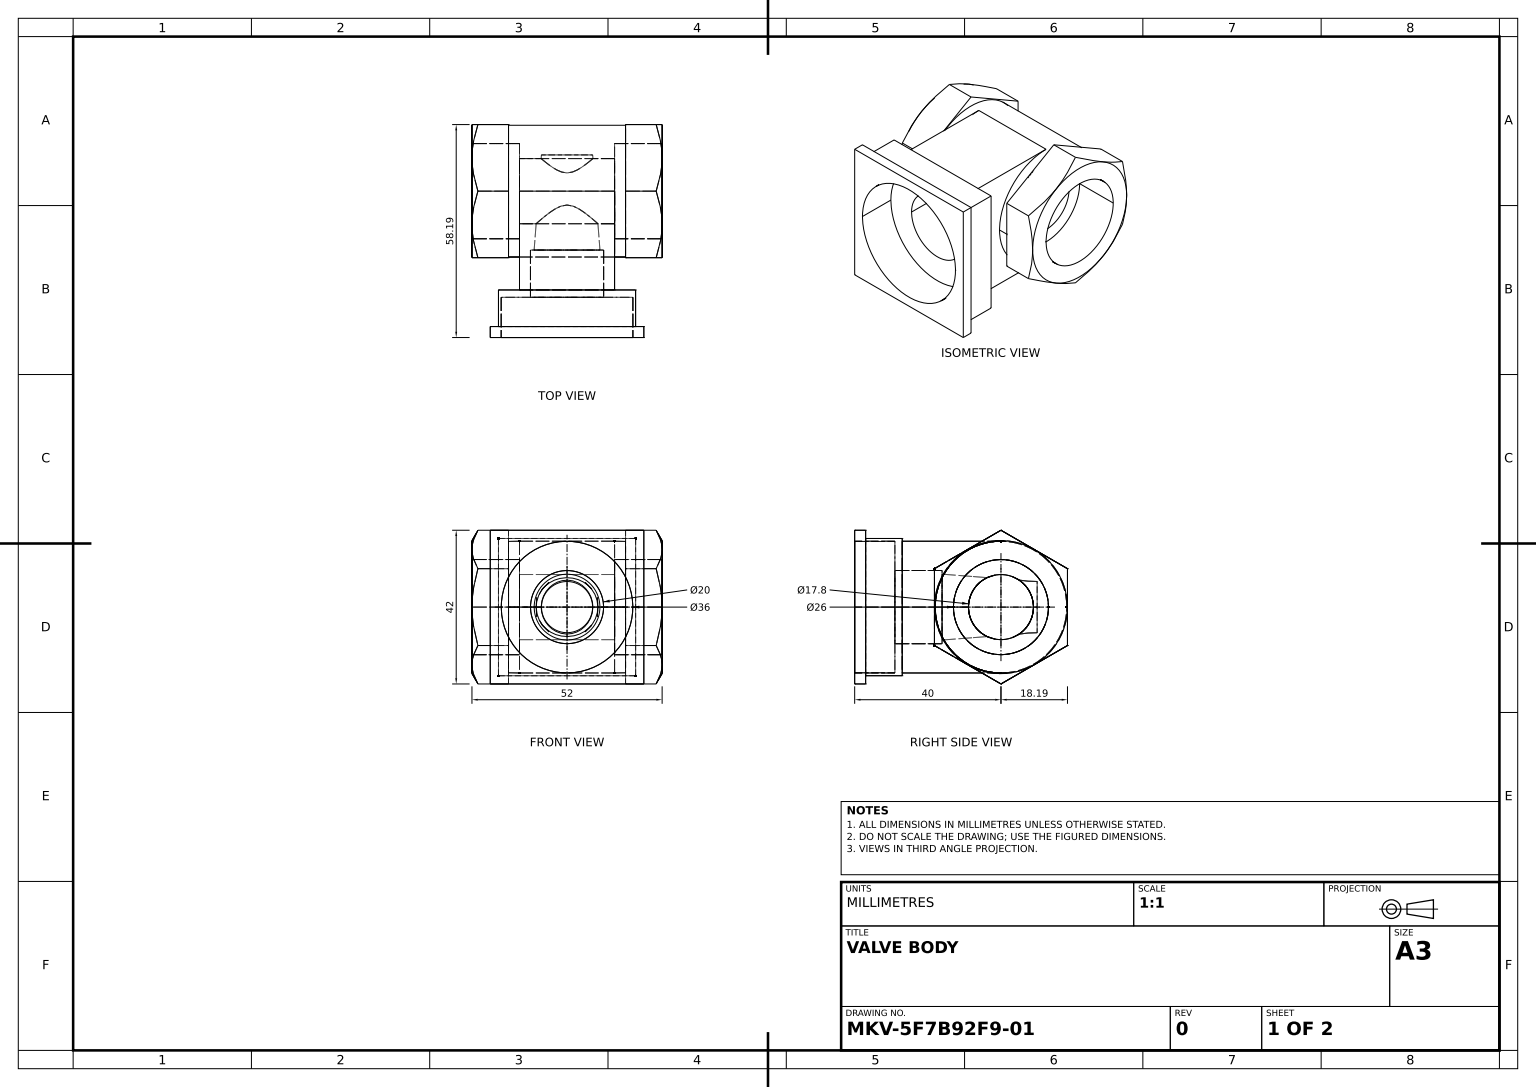
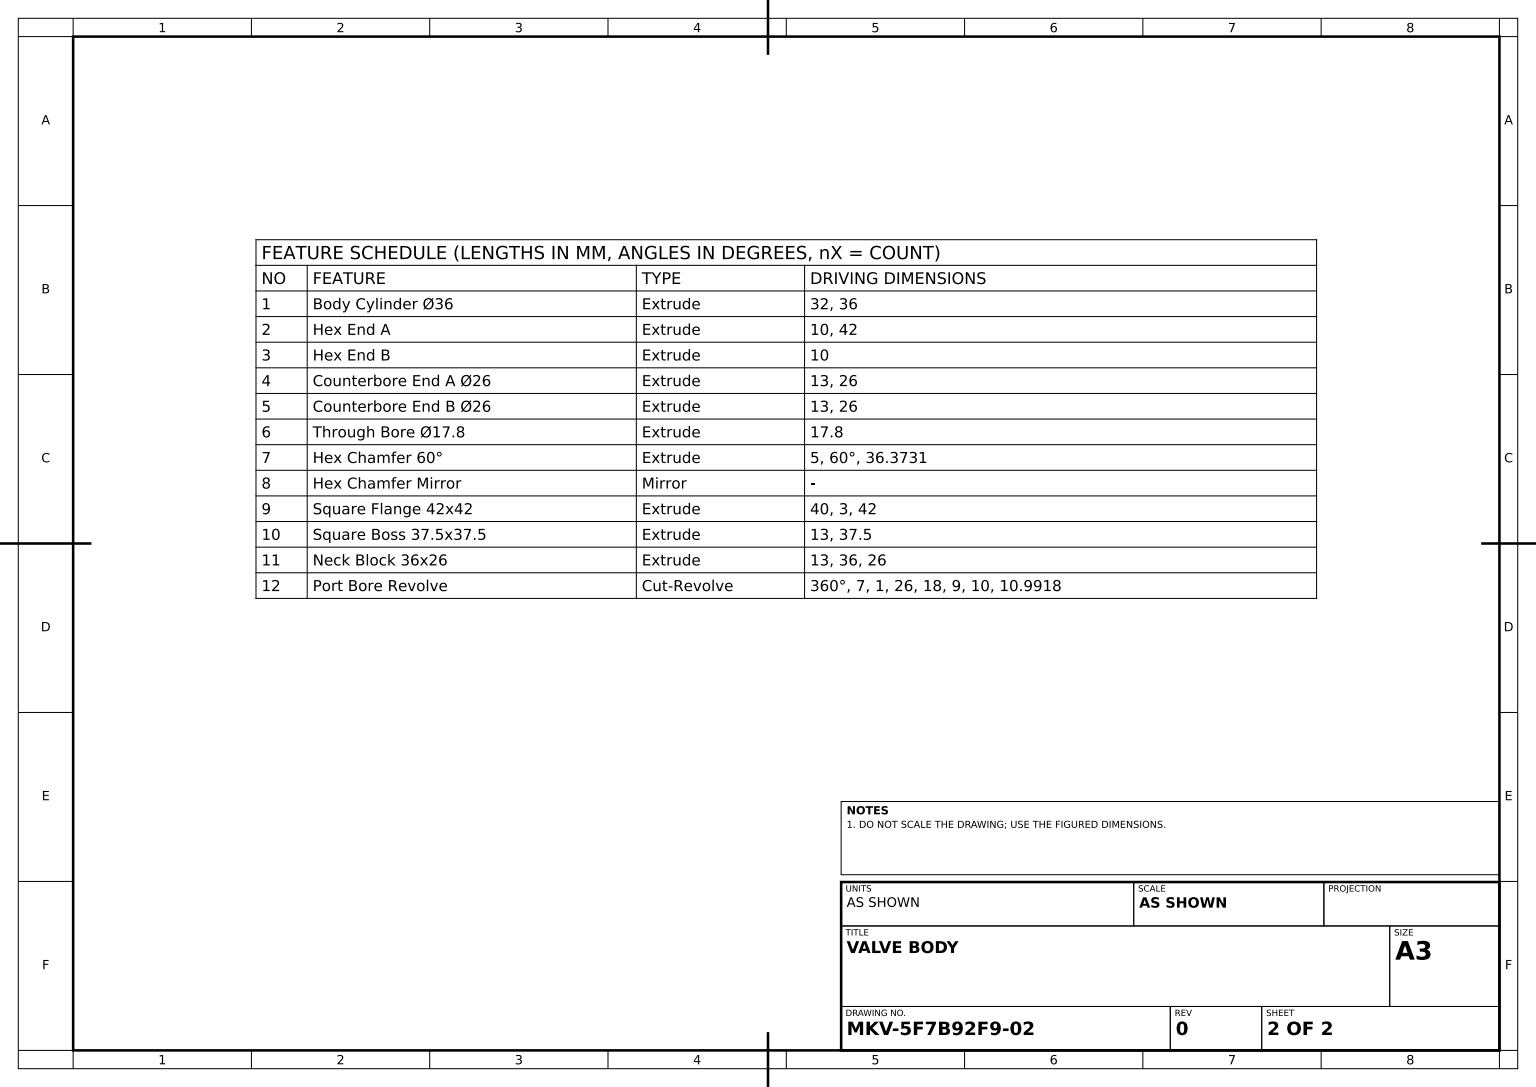
SolidWorks part; units mm, degrees
material "Plain Carbon Steel"
ref_plane "Front Plane" through (0, 0, 0) normal (0, 0, 1) x (1, 0, 0)
ref_plane "Top Plane" through (0, 0, 0) normal (0, 1, 0) x (1, 0, 0)
ref_plane "Right Plane" through (0, 0, 0) normal (1, 0, 0) x (0, 0, -1)
sketch "Body Profile Ø36" plane through (0, 0, 0) normal (1, 0, 0) x (0, 0, -1)
  circle A0 centre (0, 0) radius 18
  dimension "D1" = 36
extrude "Body Cylinder Ø36" add sketch "Body Profile Ø36" along normal mid plane 32
sketch "Hex Profile End A 42" plane through (16, 0, 0) normal (1, 0, 0) x (0, 0, -1)
  line L1 (0, 21) -> (-18.1865, 10.5)
  line L2 (-18.1865, 10.5) -> (-18.1865, -10.5)
  line L3 (-18.1865, -10.5) -> (0, -21)
  line L4 (0, -21) -> (18.1865, -10.5)
  line L5 (18.1865, -10.5) -> (18.1865, 10.5)
  line L6 (18.1865, 10.5) -> (0, 21)
  circle A0 centre (0, 0) radius 18.1865 construction
  dimension "D1" = 42
extrude "Hex End A" add sketch "Hex Profile End A 42" along normal blind 10
sketch "Hex Profile End B" plane through (-16, 0, 0) normal (-1, 0, 0) x (0, 0, 1)
  line L6 (18.1865, 10.5) -> (0, 21)
  line L7 (18.1865, -10.5) -> (18.1865, 10.5)
  line L8 (0, -21) -> (18.1865, -10.5)
  line L9 (-18.1865, -10.5) -> (0, -21)
  line L10 (-18.1865, 10.5) -> (-18.1865, -10.5)
  line L11 (0, 21) -> (-18.1865, 10.5)
  line L12 (18.1865, 10.5) -> (0, 21)
  line L13 (18.1865, -10.5) -> (18.1865, 10.5)
  line L14 (0, -21) -> (18.1865, -10.5)
  line L15 (-18.1865, -10.5) -> (0, -21)
  line L16 (-18.1865, 10.5) -> (-18.1865, -10.5)
  line L17 (0, 21) -> (-18.1865, 10.5)
  dimension "D1" = 0
extrude "Hex End B" add sketch "Hex Profile End B" along normal blind 10
sketch "Counterbore Profile End A Ø26" plane through (26, 0, 0) normal (1, 0, 0) x (0, 0, -1)
  circle A0 centre (0, 0) radius 13
  dimension "D1" = 26
extrude "Counterbore End A Ø26" cut sketch "Counterbore Profile End A Ø26" against normal blind 13
sketch "Counterbore Profile End B Ø26" plane through (-26, 0, 0) normal (-1, 0, 0) x (0, 0, 1)
  circle A0 centre (0, 0) radius 13
  dimension "D1" = 26
extrude "Counterbore End B Ø26" cut sketch "Counterbore Profile End B Ø26" against normal blind 13
sketch "Through Bore Profile Ø17.8" plane through (-13, 0, 0) normal (-1, 0, 0) x (0, 0, 1)
  circle A0 centre (0, 0) radius 8.9
  dimension "D1" = 17.8
extrude "Through Bore Ø17.8" cut sketch "Through Bore Profile Ø17.8" against normal through all
sketch "Hex Chamfer Profile" plane through (-26, 0, 0) normal (-1, 0, 0) x (0, 0, 1)
  circle A0 centre (0, 0) radius 18.1865
  dimension "D1" = 36.3731
extrude "Hex Chamfer 60°" cut sketch "Hex Chamfer Profile" against normal blind 5 draft 60 flip side to cut
mirror "Hex Chamfer Mirror" about plane through (0, 0, 0) normal (1, 0, 0) of "Hex Chamfer 60°"
ref_plane "Flange Face Plane" through (0, 0, 40) normal (0, 0, 1) x (1, 0, 0)
sketch "Flange Profile 42x42" plane through (0, 0, 40) normal (0, 0, 1) x (1, 0, 0)
  line L1 (-21, -21) -> (21, -21)
  line L2 (-21, -21) -> (-21, 21)
  line L3 (-21, 21) -> (21, 21)
  line L4 (21, -21) -> (21, 21)
  line L5 (-21, -21) -> (21, 21) construction
  line L6 (-21, 21) -> (21, -21) construction
  point P0 (0, 0)
  dimension "D1" = 42
  dimension "D2" = 42
extrude "Square Flange 42x42" add sketch "Flange Profile 42x42" against normal blind 3 separate body
sketch "Square Boss Profile 37.5x37.5" plane through (0, 0, 40) normal (0, 0, 1) x (1, 0, 0)
  line L1 (-18.75, -18.75) -> (18.75, -18.75)
  line L2 (-18.75, -18.75) -> (-18.75, 18.75)
  line L3 (-18.75, 18.75) -> (18.75, 18.75)
  line L4 (18.75, -18.75) -> (18.75, 18.75)
  line L5 (-18.75, -18.75) -> (18.75, 18.75) construction
  line L6 (-18.75, 18.75) -> (18.75, -18.75) construction
  point P0 (0, 0)
  dimension "D1" = 37.5
  dimension "D2" = 37.5
extrude "Square Boss 37.5x37.5" add sketch "Square Boss Profile 37.5x37.5" against normal blind 13
sketch "Neck Block Profile 36x26" plane through (0, 0, 40) normal (0, 0, 1) x (1, 0, 0)
  line L1 (-13, -18) -> (13, -18)
  line L2 (-13, -18) -> (-13, 18)
  line L3 (-13, 18) -> (13, 18)
  line L4 (13, -18) -> (13, 18)
  line L5 (-13, -18) -> (13, 18) construction
  line L6 (-13, 18) -> (13, -18) construction
  point P0 (0, 0)
  dimension "D1" = 36
  dimension "D2" = 26
extrude "Neck Block 36x26" add sketch "Neck Block Profile 36x26" against normal up to body
sketch "Port Bore Profile" plane through (0, 0, 0) normal (0, 1, 0) x (1, 0, 0)
  line L0 (0, -40) -> (0, 9.9)
  line L1 (21, -40) -> (-21, -40) construction
  line L2 (0, 9.9) -> (7, 9.9)
  line L3 (7, 9.9) -> (9, -16.1)
  line L4 (9, -16.1) -> (10, -16.1)
  line L5 (10, -16.1) -> (10, -29.0082)
  line L6 (10, -29.0082) -> (18, -29.0082)
  line L7 (18, -29.0082) -> (18, -40)
  line L8 (13, 8.9) -> (-13, 8.9) construction
  line L9 (0, -40) -> (18, -40)
  dimension "D1" = 7
  dimension "D2" = 1
  dimension "D3" = 26
  dimension "D4" = 9
  dimension "D5" = 10
  dimension "D6" = 18
  dimension "D7" = 10.9918
revolve "Port Bore Revolve" cut sketch "Port Bore Profile" angle 360 about L0
